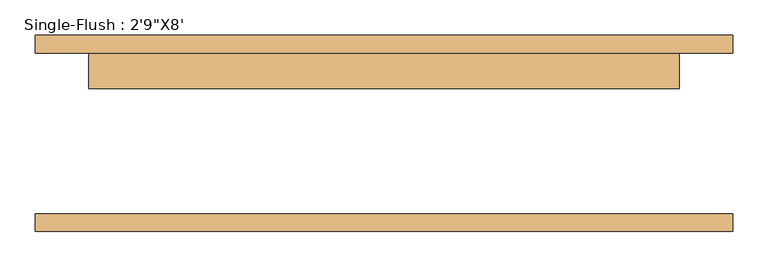
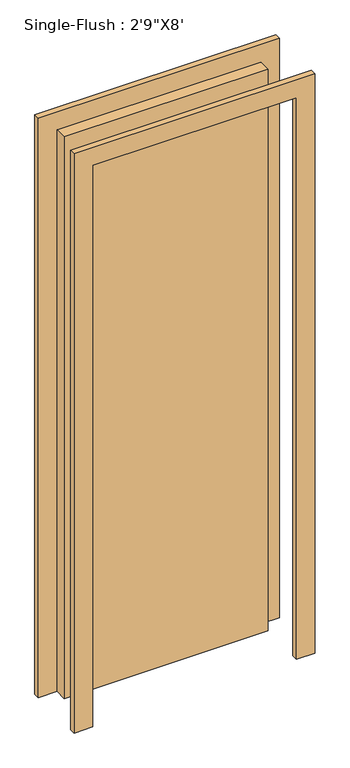
"""IFC4 building model written with IfcOpenShell, lengths in millimetres: door geometry."""

from ifc_helpers import new_model, si_unit, frame, origin, origin_with_axes, place, context, project, spatial, polyline, outline, extrude, source, transform, mapped, element, save


def door_4b41b0c1(model_context):
    return source(origin(), model_context, "Body", "SweptSolid", [
        extrude(outline(polyline([(2514.6, -495.3), (0.0, -495.3), (0.0, -419.1), (2438.4, -419.1), (2438.4, 419.1), (0.0, 419.1), (0.0, 495.3), (2514.6, 495.3), (2514.6, -495.3)])), frame((0.0, 114.3, 0.0), z_axis=(0.0, 1.0, 0.0), x_axis=(0.0, 0.0, 1.0)), (0.0, 0.0, 1.0), 25.4),
        extrude(outline(polyline([(2514.6, 495.3), (2514.6, -495.3), (0.0, -495.3), (0.0, -419.1), (2438.4, -419.1), (2438.4, 419.1), (0.0, 419.1), (0.0, 495.3), (2514.6, 495.3)])), frame((0.0, -139.7, 0.0), z_axis=(0.0, 1.0, 0.0), x_axis=(0.0, 0.0, 1.0)), (0.0, 0.0, 1.0), 25.4),
        extrude(outline(polyline([(419.1, 63.5), (-419.1, 63.5), (-419.1, 114.3), (419.1, 114.3), (419.1, 63.5)])), origin_with_axes(), (0.0, 0.0, 1.0), 2438.4),
    ])


if __name__ == "__main__":
    model = new_model("IFC4")
    model_context = context("Model", 3, world=origin())
    ifc_project = project(units=[si_unit("LENGTHUNIT", "METRE", prefix="MILLI")], contexts=[model_context])
    site = spatial("IfcSite", under=ifc_project)
    building = spatial("IfcBuilding", under=site)
    placement = place(None, origin())
    door_shape = door_4b41b0c1(model_context)
    element("IfcDoor", 1, ObjectType="Single-Flush : 2'9\"X8'", at=placement, inside=building, context=model_context, shape_type="MappedRepresentation", body=[
        mapped(door_shape, transform((0.0, 0.0, 0.0), x_axis=(1.0, 0.0, 0.0), y_axis=(0.0, 1.0, 0.0), z_axis=(0.0, 0.0, 1.0))),
    ])
    save(model, "model.ifc")

# Revit data of these elements
# Type "Single-Flush : 2'9\"X8'"
#   Type Mark = "9"
#   Construction Type Id = "MDOOR"
#   Assembly Code = "C1020"
#   Analytic Construction = "Metal"
#   Thickness = 0' - 2"
#   Heat Transfer Coefficient (U) = 0.651978 BTU/(h·ft²·°F)
#   Height = 8' - 0"
#   Trim Projection Ext = 0' - 1"
#   Trim Projection Int = 0' - 1"
#   Trim Width = 0' - 3"
#   Width = 2' - 9"
#   Define Thermal Properties by = 1
#   Door Material = Door - Panel
#   Frame Material = Door - Frame
#   Visual Light Transmittance = 0
#   Solar Heat Gain Coefficient = 0
#   Function = (empty or 0)
#   Wall Closure = (empty or 0)
# Element 1 (IfcDoor, "Single-Flush : 2'9\"X8'")
#   Materials on its faces: "Door - Frame", "Door - Panel"
# Materials
#   "Door - Panel": class "Wood", colour RGB 210 159 95, transparency 0, Cost = 0
#   "Door - Frame": colour RGB 118 70 51, transparency 0, Cost = 0
